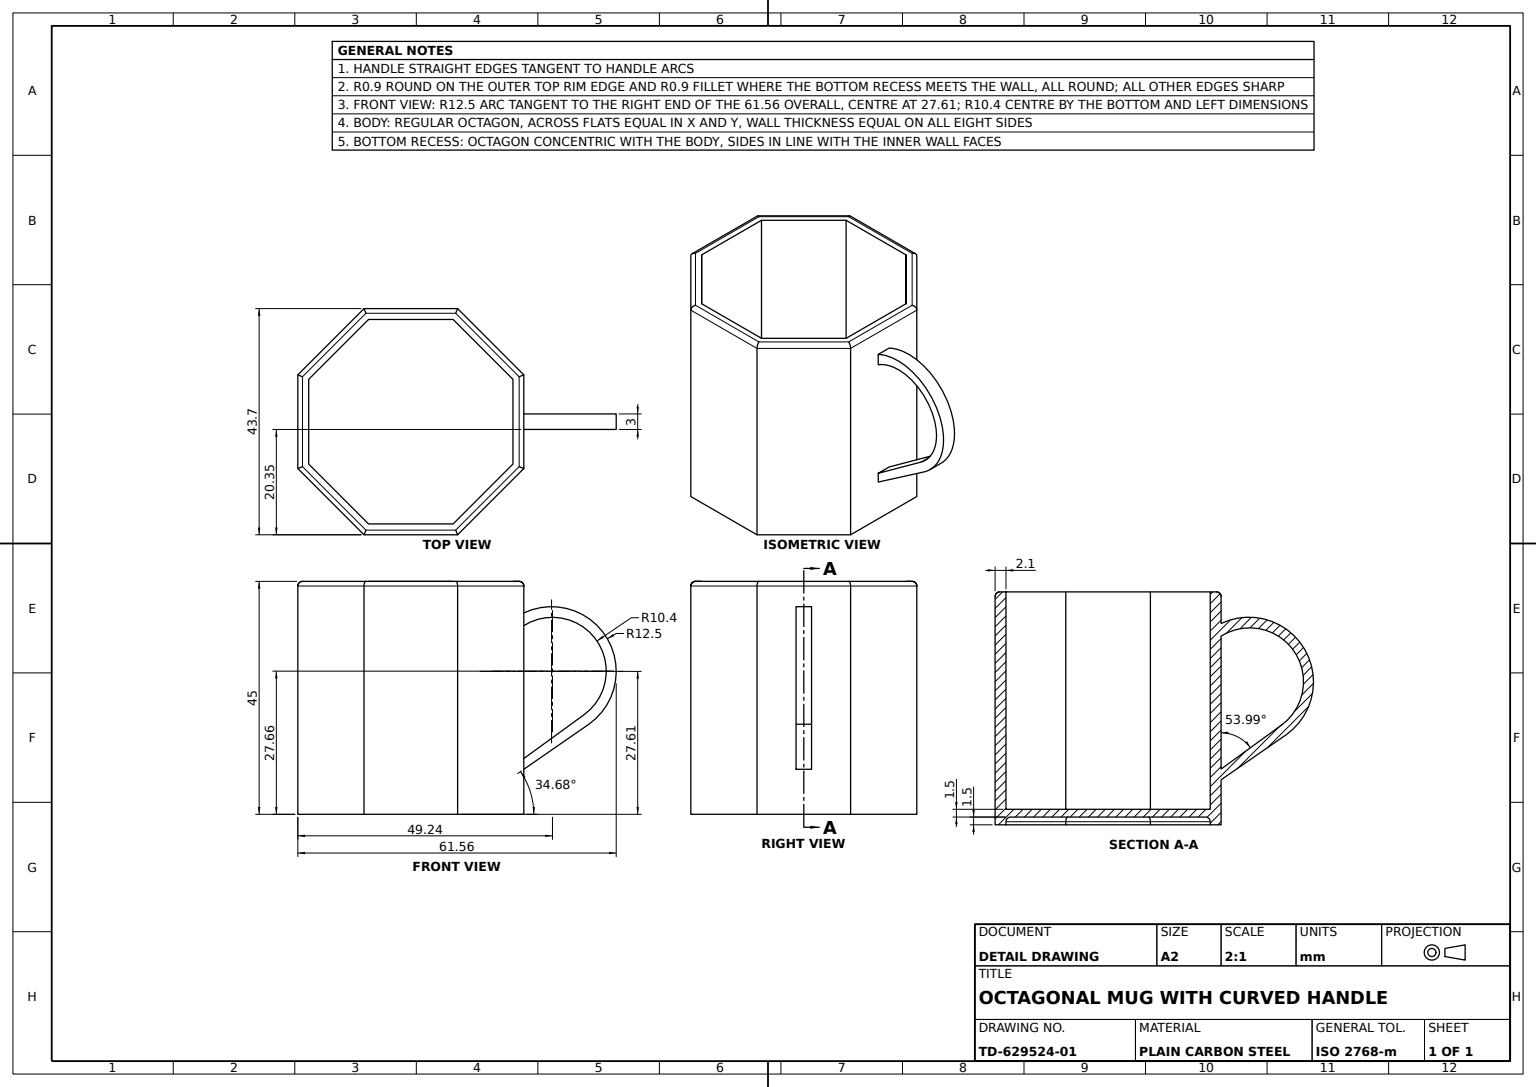
SolidWorks part; units mm, degrees
material "Plain Carbon Steel"
ref_plane "Front Plane" through (0, 0, 0) normal (0, 0, 1) x (1, 0, 0)
ref_plane "Top Plane" through (0, 0, 0) normal (0, 1, 0) x (1, 0, 0)
ref_plane "Right Plane" through (0, 0, 0) normal (1, 0, 0) x (0, 0, -1)
sketch "Octagon Wall Profile" plane through (0, 0, 0) normal (0, 1, 0) x (1, 0, 0)
  line L0 (-19.7486, 8.1802) -> (-19.7486, -8.1802)
  line L1 (21.8486, -9.05) -> (21.8486, 9.05)
  line L2 (21.8486, 9.05) -> (9.05, 21.8486)
  line L3 (9.05, 21.8486) -> (-9.05, 21.8486)
  line L4 (-9.05, 21.8486) -> (-21.8486, 9.05)
  line L5 (-21.8486, 9.05) -> (-21.8486, -9.05)
  line L6 (-21.8486, -9.05) -> (-9.05, -21.8486)
  line L7 (-9.05, -21.8486) -> (9.05, -21.8486)
  line L8 (9.05, -21.8486) -> (21.8486, -9.05)
  line L9 (-19.7486, -8.1802) -> (-8.1802, -19.7486)
  line L10 (-8.1802, -19.7486) -> (8.1802, -19.7486)
  line L11 (8.1802, -19.7486) -> (19.7486, -8.1802)
  line L12 (19.7486, -8.1802) -> (19.7486, 8.1802)
  line L13 (19.7486, 8.1802) -> (8.1802, 19.7486)
  line L14 (8.1802, 19.7486) -> (-8.1802, 19.7486)
  line L15 (-8.1802, 19.7486) -> (-19.7486, 8.1802)
  circle A0 centre (0, 0) radius 21.8486 construction
  dimension "D1" = 18.1
  dimension "D2" = 2.1
extrude "Octagon Wall 45mm" add sketch "Octagon Wall Profile" along normal blind 45
sketch "Bottom Plate Profile" plane through (0, 0, 0) normal (0, -1, 0) x (1, 0, 0)
  line L1 (19.7486, -8.1802) -> (19.7486, 8.1802)
  line L2 (19.7486, 8.1802) -> (8.1802, 19.7486)
  line L3 (8.1802, 19.7486) -> (-8.1802, 19.7486)
  line L4 (-8.1802, 19.7486) -> (-19.7486, 8.1802)
  line L5 (-19.7486, 8.1802) -> (-19.7486, -8.1802)
  line L6 (-19.7486, -8.1802) -> (-8.1802, -19.7486)
  line L7 (-8.1802, -19.7486) -> (8.1802, -19.7486)
  line L8 (8.1802, -19.7486) -> (19.7486, -8.1802)
  circle A0 centre (0, 0) radius 19.7486 construction
  dimension "D1" = 16.3603
extrude "Bottom Plate 1.5mm" add sketch "Bottom Plate Profile" along normal blind 1.5 from offset 3 offset against normal yes
fillet "Bottom Plate Fillet R0.9" radius 0.9 8 edges at (0, 1.5, 19.7486) (-13.9644, 1.5, 13.9644) (-19.7486, 1.5, 0) (-13.9644, 1.5, -13.9644) (0, 1.5, -19.7486) (13.9644, 1.5, -13.9644) (19.7486, 1.5, 0) (13.9644, 1.5, 13.9644)
sketch "Handle Profile" plane through (0, 0, 0) normal (0, 0, 1) x (1, 0, 0)
  line L0 (21.8486, 45) -> (21.8486, 0) construction
  line L1 (21.8486, 38.9002) -> (21.8486, 0)
  line L2 (33.5043, 19.2436) -> (21.8486, 10.7718)
  line L3 (21.8486, 8.6979) -> (34.4305, 17.4035)
  arc A0 (33.5043, 19.2436) -> (21.8486, 36.4572) centre (27.3896, 27.6562) ccw
  arc A1 (34.4305, 17.4035) -> (21.8486, 38.9002) centre (27.2154, 27.6109) ccw
  dimension "D2" = 15.3
  dimension "D3" = 10.4
  dimension "D4" = 12.5
  dimension "D1" = 27.3896
  dimension "D5" = 10.7718
  dimension "D6" = 27.6109
  dimension "D7" = 8.6979
  dimension "D8" = 27.6562
  dimension "D9" = 27.2154
extrude "Handle 3mm" add sketch "Handle Profile" along normal mid plane 3 contours L3 A1 L1 A0 L2
fillet "Wall Edge Fillet R0.9" radius 0.9 8 edges at (15.4493, 45, 15.4493) (0, 45, 21.8486) (-15.4493, 45, 15.4493) (-21.8486, 45, 0) (-15.4493, 45, -15.4493) (0, 45, -21.8486) (15.4493, 45, -15.4493) (21.8486, 45, 0)
